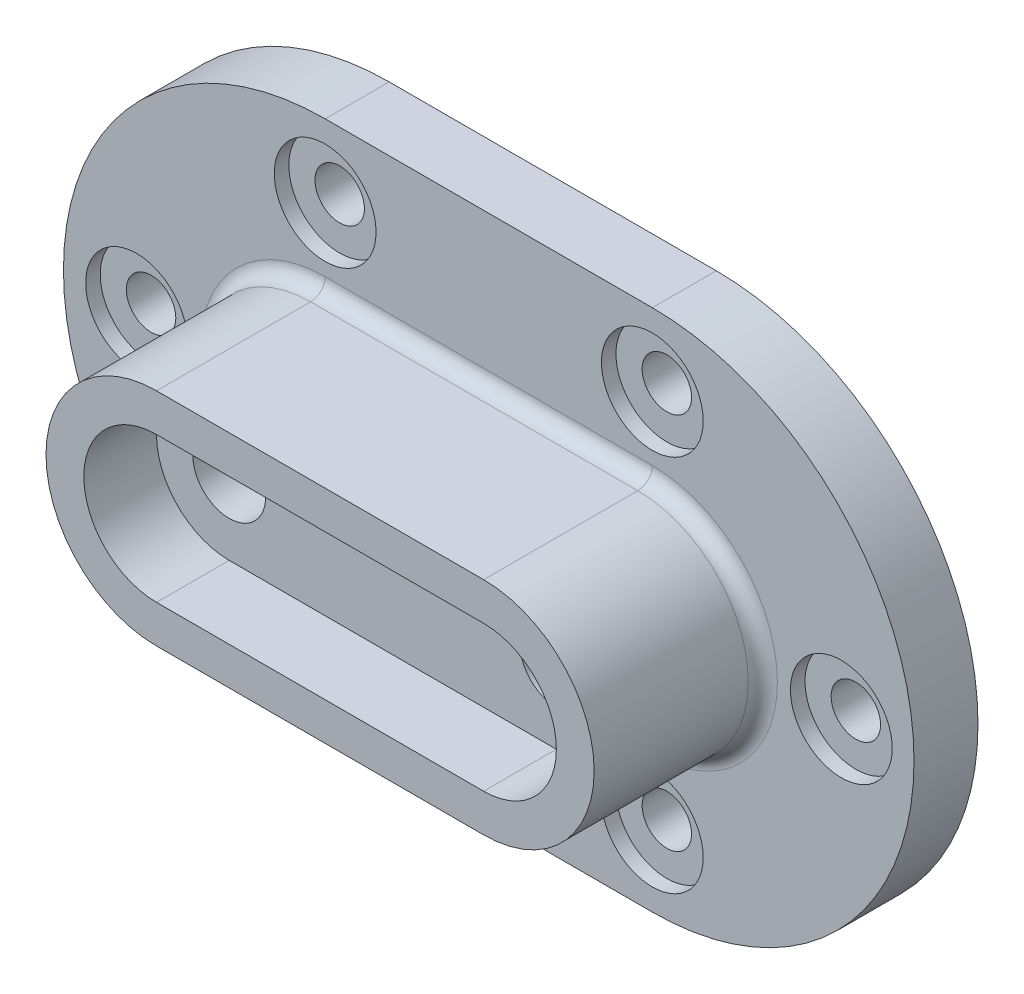
ISO-10303-21;
HEADER;
FILE_DESCRIPTION(('STEP AP214'),'2;1');
FILE_NAME('part.step','',(''),(''),'','','');
FILE_SCHEMA(('AUTOMOTIVE_DESIGN { 1 0 10303 214 1 1 1 1 }'));
ENDSEC;
DATA;
#1=APPLICATION_CONTEXT('core data for automotive mechanical design processes');
#2=APPLICATION_PROTOCOL_DEFINITION('international standard','automotive_design',2000,#1);
#3=PRODUCT_CONTEXT('',#1,'mechanical');
#4=PRODUCT('Part','Part','',(#3));
#5=PRODUCT_RELATED_PRODUCT_CATEGORY('part','',(#4));
#6=PRODUCT_DEFINITION_FORMATION('','',#4);
#7=PRODUCT_DEFINITION_CONTEXT('part definition',#1,'design');
#8=PRODUCT_DEFINITION('design','',#6,#7);
#9=PRODUCT_DEFINITION_SHAPE('','',#8);
#10=(LENGTH_UNIT() NAMED_UNIT(*) SI_UNIT(.MILLI.,.METRE.));
#11=(NAMED_UNIT(*) PLANE_ANGLE_UNIT() SI_UNIT($,.RADIAN.));
#12=(NAMED_UNIT(*) SI_UNIT($,.STERADIAN.) SOLID_ANGLE_UNIT());
#13=UNCERTAINTY_MEASURE_WITH_UNIT(LENGTH_MEASURE(1.E-05),#10,'distance_accuracy_value','');
#14=(GEOMETRIC_REPRESENTATION_CONTEXT(3) GLOBAL_UNCERTAINTY_ASSIGNED_CONTEXT((#13)) GLOBAL_UNIT_ASSIGNED_CONTEXT((#10,
#11,#12)) REPRESENTATION_CONTEXT('',''));
#15=CARTESIAN_POINT('',(0.,0.,0.));
#16=DIRECTION('',(0.,0.,1.));
#17=DIRECTION('',(1.,0.,0.));
#18=AXIS2_PLACEMENT_3D('',#15,#16,#17);
#19=CARTESIAN_POINT('',(-11.25,13.,-0.6));
#20=DIRECTION('',(0.,0.,1.));
#21=DIRECTION('',(1.,0.,0.));
#22=AXIS2_PLACEMENT_3D('',#19,#20,#21);
#23=CYLINDRICAL_SURFACE('',#22,1.7);
#24=CARTESIAN_POINT('',(-11.25,13.,0.));
#25=DIRECTION('',(0.,0.,1.));
#26=DIRECTION('',(1.,0.,0.));
#27=AXIS2_PLACEMENT_3D('',#24,#25,#26);
#28=CIRCLE('',#27,1.7);
#29=CARTESIAN_POINT('',(-9.55000000000004,13.,0.));
#30=VERTEX_POINT('',#29);
#31=EDGE_CURVE('E240',#30,#30,#28,.T.);
#32=ORIENTED_EDGE('',*,*,#31,.F.);
#33=EDGE_LOOP('',(#32));
#34=FACE_BOUND('',#33,.T.);
#35=CARTESIAN_POINT('',(-11.25,13.,3.4));
#36=DIRECTION('',(0.,0.,1.));
#37=DIRECTION('',(1.,0.,0.));
#38=AXIS2_PLACEMENT_3D('',#35,#36,#37);
#39=CIRCLE('',#38,1.7);
#40=CARTESIAN_POINT('',(-9.55000000000004,13.,3.4));
#41=VERTEX_POINT('',#40);
#42=EDGE_CURVE('E243',#41,#41,#39,.F.);
#43=ORIENTED_EDGE('',*,*,#42,.F.);
#44=EDGE_LOOP('',(#43));
#45=FACE_BOUND('',#44,.T.);
#46=ADVANCED_FACE('F39',(#34,#45),#23,.F.);
#47=CARTESIAN_POINT('',(11.2499999999999,13.,-0.6));
#48=DIRECTION('',(0.,0.,1.));
#49=DIRECTION('',(1.,0.,0.));
#50=AXIS2_PLACEMENT_3D('',#47,#48,#49);
#51=CYLINDRICAL_SURFACE('',#50,1.7);
#52=CARTESIAN_POINT('',(11.2499999999999,13.,0.));
#53=DIRECTION('',(0.,0.,1.));
#54=DIRECTION('',(1.,0.,0.));
#55=AXIS2_PLACEMENT_3D('',#52,#53,#54);
#56=CIRCLE('',#55,1.7);
#57=CARTESIAN_POINT('',(12.9499999999999,13.,0.));
#58=VERTEX_POINT('',#57);
#59=EDGE_CURVE('E238',#58,#58,#56,.T.);
#60=ORIENTED_EDGE('',*,*,#59,.F.);
#61=EDGE_LOOP('',(#60));
#62=FACE_BOUND('',#61,.T.);
#63=CARTESIAN_POINT('',(11.2499999999999,13.,3.4));
#64=DIRECTION('',(0.,0.,1.));
#65=DIRECTION('',(1.,0.,0.));
#66=AXIS2_PLACEMENT_3D('',#63,#64,#65);
#67=CIRCLE('',#66,1.7);
#68=CARTESIAN_POINT('',(12.9499999999999,13.,3.4));
#69=VERTEX_POINT('',#68);
#70=EDGE_CURVE('E268',#69,#69,#67,.F.);
#71=ORIENTED_EDGE('',*,*,#70,.F.);
#72=EDGE_LOOP('',(#71));
#73=FACE_BOUND('',#72,.T.);
#74=ADVANCED_FACE('F399',(#62,#73),#51,.F.);
#75=CARTESIAN_POINT('',(24.25,0.,-0.6));
#76=DIRECTION('',(0.,0.,1.));
#77=DIRECTION('',(1.,0.,0.));
#78=AXIS2_PLACEMENT_3D('',#75,#76,#77);
#79=CYLINDRICAL_SURFACE('',#78,1.7);
#80=CARTESIAN_POINT('',(24.25,0.,0.));
#81=DIRECTION('',(0.,0.,1.));
#82=DIRECTION('',(1.,0.,0.));
#83=AXIS2_PLACEMENT_3D('',#80,#81,#82);
#84=CIRCLE('',#83,1.7);
#85=CARTESIAN_POINT('',(25.95,0.,0.));
#86=VERTEX_POINT('',#85);
#87=EDGE_CURVE('E242',#86,#86,#84,.T.);
#88=ORIENTED_EDGE('',*,*,#87,.F.);
#89=EDGE_LOOP('',(#88));
#90=FACE_BOUND('',#89,.T.);
#91=CARTESIAN_POINT('',(24.25,0.,3.4));
#92=DIRECTION('',(0.,0.,1.));
#93=DIRECTION('',(1.,0.,0.));
#94=AXIS2_PLACEMENT_3D('',#91,#92,#93);
#95=CIRCLE('',#94,1.7);
#96=CARTESIAN_POINT('',(25.95,0.,3.4));
#97=VERTEX_POINT('',#96);
#98=EDGE_CURVE('E264',#97,#97,#95,.F.);
#99=ORIENTED_EDGE('',*,*,#98,.F.);
#100=EDGE_LOOP('',(#99));
#101=FACE_BOUND('',#100,.T.);
#102=ADVANCED_FACE('F401',(#90,#101),#79,.F.);
#103=CARTESIAN_POINT('',(11.2500000000001,-13.,-0.6));
#104=DIRECTION('',(0.,0.,1.));
#105=DIRECTION('',(1.,0.,0.));
#106=AXIS2_PLACEMENT_3D('',#103,#104,#105);
#107=CYLINDRICAL_SURFACE('',#106,1.7);
#108=CARTESIAN_POINT('',(11.2500000000001,-13.,0.));
#109=DIRECTION('',(0.,0.,1.));
#110=DIRECTION('',(1.,0.,0.));
#111=AXIS2_PLACEMENT_3D('',#108,#109,#110);
#112=CIRCLE('',#111,1.7);
#113=CARTESIAN_POINT('',(12.9500000000001,-13.,0.));
#114=VERTEX_POINT('',#113);
#115=EDGE_CURVE('E246',#114,#114,#112,.T.);
#116=ORIENTED_EDGE('',*,*,#115,.F.);
#117=EDGE_LOOP('',(#116));
#118=FACE_BOUND('',#117,.T.);
#119=CARTESIAN_POINT('',(11.2500000000001,-13.,3.4));
#120=DIRECTION('',(0.,0.,1.));
#121=DIRECTION('',(1.,0.,0.));
#122=AXIS2_PLACEMENT_3D('',#119,#120,#121);
#123=CIRCLE('',#122,1.7);
#124=CARTESIAN_POINT('',(12.9500000000001,-13.,3.4));
#125=VERTEX_POINT('',#124);
#126=EDGE_CURVE('E265',#125,#125,#123,.F.);
#127=ORIENTED_EDGE('',*,*,#126,.F.);
#128=EDGE_LOOP('',(#127));
#129=FACE_BOUND('',#128,.T.);
#130=ADVANCED_FACE('F413',(#118,#129),#107,.F.);
#131=CARTESIAN_POINT('',(-11.2499999999999,-13.,-0.6));
#132=DIRECTION('',(0.,0.,1.));
#133=DIRECTION('',(1.,0.,0.));
#134=AXIS2_PLACEMENT_3D('',#131,#132,#133);
#135=CYLINDRICAL_SURFACE('',#134,1.7);
#136=CARTESIAN_POINT('',(-11.2499999999999,-13.,0.));
#137=DIRECTION('',(0.,0.,1.));
#138=DIRECTION('',(1.,0.,0.));
#139=AXIS2_PLACEMENT_3D('',#136,#137,#138);
#140=CIRCLE('',#139,1.7);
#141=CARTESIAN_POINT('',(-9.54999999999986,-13.,0.));
#142=VERTEX_POINT('',#141);
#143=EDGE_CURVE('E247',#142,#142,#140,.T.);
#144=ORIENTED_EDGE('',*,*,#143,.F.);
#145=EDGE_LOOP('',(#144));
#146=FACE_BOUND('',#145,.T.);
#147=CARTESIAN_POINT('',(-11.2499999999999,-13.,3.4));
#148=DIRECTION('',(0.,0.,1.));
#149=DIRECTION('',(1.,0.,0.));
#150=AXIS2_PLACEMENT_3D('',#147,#148,#149);
#151=CIRCLE('',#150,1.7);
#152=CARTESIAN_POINT('',(-9.54999999999986,-13.,3.4));
#153=VERTEX_POINT('',#152);
#154=EDGE_CURVE('E256',#153,#153,#151,.F.);
#155=ORIENTED_EDGE('',*,*,#154,.F.);
#156=EDGE_LOOP('',(#155));
#157=FACE_BOUND('',#156,.T.);
#158=ADVANCED_FACE('F407',(#146,#157),#135,.F.);
#159=CARTESIAN_POINT('',(-24.2220429598138,0.,-0.6));
#160=DIRECTION('',(0.,0.,1.));
#161=DIRECTION('',(1.,0.,0.));
#162=AXIS2_PLACEMENT_3D('',#159,#160,#161);
#163=CYLINDRICAL_SURFACE('',#162,1.7);
#164=CARTESIAN_POINT('',(-24.2220429598138,0.,0.));
#165=DIRECTION('',(0.,0.,1.));
#166=DIRECTION('',(1.,0.,0.));
#167=AXIS2_PLACEMENT_3D('',#164,#165,#166);
#168=CIRCLE('',#167,1.7);
#169=CARTESIAN_POINT('',(-22.5220429598138,0.,0.));
#170=VERTEX_POINT('',#169);
#171=EDGE_CURVE('E178',#170,#170,#168,.T.);
#172=ORIENTED_EDGE('',*,*,#171,.F.);
#173=EDGE_LOOP('',(#172));
#174=FACE_BOUND('',#173,.T.);
#175=CARTESIAN_POINT('',(-24.2220429598138,0.,3.4));
#176=DIRECTION('',(0.,0.,1.));
#177=DIRECTION('',(1.,0.,0.));
#178=AXIS2_PLACEMENT_3D('',#175,#176,#177);
#179=CIRCLE('',#178,1.7);
#180=CARTESIAN_POINT('',(-22.5220429598138,0.,3.4));
#181=VERTEX_POINT('',#180);
#182=EDGE_CURVE('E254',#181,#181,#179,.F.);
#183=ORIENTED_EDGE('',*,*,#182,.F.);
#184=EDGE_LOOP('',(#183));
#185=FACE_BOUND('',#184,.T.);
#186=ADVANCED_FACE('F470',(#174,#185),#163,.F.);
#187=CARTESIAN_POINT('',(-11.25,0.,4.4));
#188=DIRECTION('',(0.,0.,-1.));
#189=DIRECTION('',(-1.,0.,0.));
#190=AXIS2_PLACEMENT_3D('',#187,#188,#189);
#191=CYLINDRICAL_SURFACE('',#190,18.);
#192=CARTESIAN_POINT('',(-11.25,0.,0.));
#193=DIRECTION('',(0.,0.,1.));
#194=DIRECTION('',(1.,0.,0.));
#195=AXIS2_PLACEMENT_3D('',#192,#193,#194);
#196=CIRCLE('',#195,18.);
#197=CARTESIAN_POINT('',(-11.25,18.,0.));
#198=VERTEX_POINT('',#197);
#199=CARTESIAN_POINT('',(-11.25,-18.,0.));
#200=VERTEX_POINT('',#199);
#201=EDGE_CURVE('E206',#198,#200,#196,.T.);
#202=ORIENTED_EDGE('',*,*,#201,.T.);
#203=DIRECTION('',(0.,0.,-1.));
#204=VECTOR('',#203,1.);
#205=CARTESIAN_POINT('',(-11.25,-18.,4.4));
#206=LINE('',#205,#204);
#207=CARTESIAN_POINT('',(-11.25,-18.,4.4));
#208=VERTEX_POINT('',#207);
#209=EDGE_CURVE('E235',#208,#200,#206,.T.);
#210=ORIENTED_EDGE('',*,*,#209,.F.);
#211=CARTESIAN_POINT('',(-11.25,0.,4.4));
#212=DIRECTION('',(0.,0.,1.));
#213=DIRECTION('',(1.,0.,0.));
#214=AXIS2_PLACEMENT_3D('',#211,#212,#213);
#215=CIRCLE('',#214,18.);
#216=CARTESIAN_POINT('',(-11.25,18.,4.4));
#217=VERTEX_POINT('',#216);
#218=EDGE_CURVE('E210',#217,#208,#215,.T.);
#219=ORIENTED_EDGE('',*,*,#218,.F.);
#220=DIRECTION('',(0.,0.,-1.));
#221=VECTOR('',#220,1.);
#222=CARTESIAN_POINT('',(-11.25,18.,4.4));
#223=LINE('',#222,#221);
#224=EDGE_CURVE('E220',#217,#198,#223,.T.);
#225=ORIENTED_EDGE('',*,*,#224,.T.);
#226=EDGE_LOOP('',(#202,#210,#219,#225));
#227=FACE_BOUND('',#226,.T.);
#228=ADVANCED_FACE('F366',(#227),#191,.T.);
#229=CARTESIAN_POINT('',(-11.25,-18.,4.4));
#230=DIRECTION('',(0.,1.,0.));
#231=DIRECTION('',(-1.,0.,0.));
#232=AXIS2_PLACEMENT_3D('',#229,#230,#231);
#233=PLANE('',#232);
#234=DIRECTION('',(1.,0.,0.));
#235=VECTOR('',#234,1.);
#236=CARTESIAN_POINT('',(-11.25,-18.,0.));
#237=LINE('',#236,#235);
#238=CARTESIAN_POINT('',(11.25,-18.,0.));
#239=VERTEX_POINT('',#238);
#240=EDGE_CURVE('E219',#200,#239,#237,.T.);
#241=ORIENTED_EDGE('',*,*,#240,.T.);
#242=DIRECTION('',(0.,0.,-1.));
#243=VECTOR('',#242,1.);
#244=CARTESIAN_POINT('',(11.25,-18.,4.4));
#245=LINE('',#244,#243);
#246=CARTESIAN_POINT('',(11.25,-18.,4.4));
#247=VERTEX_POINT('',#246);
#248=EDGE_CURVE('E229',#247,#239,#245,.T.);
#249=ORIENTED_EDGE('',*,*,#248,.F.);
#250=DIRECTION('',(1.,0.,0.));
#251=VECTOR('',#250,1.);
#252=CARTESIAN_POINT('',(-11.25,-18.,4.4));
#253=LINE('',#252,#251);
#254=EDGE_CURVE('E209',#208,#247,#253,.T.);
#255=ORIENTED_EDGE('',*,*,#254,.F.);
#256=ORIENTED_EDGE('',*,*,#209,.T.);
#257=EDGE_LOOP('',(#241,#249,#255,#256));
#258=FACE_BOUND('',#257,.T.);
#259=ADVANCED_FACE('F371',(#258),#233,.F.);
#260=CARTESIAN_POINT('',(11.25,0.,4.4));
#261=DIRECTION('',(0.,0.,-1.));
#262=DIRECTION('',(-1.,0.,0.));
#263=AXIS2_PLACEMENT_3D('',#260,#261,#262);
#264=CYLINDRICAL_SURFACE('',#263,18.);
#265=CARTESIAN_POINT('',(11.25,0.,0.));
#266=DIRECTION('',(0.,0.,1.));
#267=DIRECTION('',(1.,0.,0.));
#268=AXIS2_PLACEMENT_3D('',#265,#266,#267);
#269=CIRCLE('',#268,18.);
#270=CARTESIAN_POINT('',(11.25,18.,0.));
#271=VERTEX_POINT('',#270);
#272=EDGE_CURVE('E225',#239,#271,#269,.T.);
#273=ORIENTED_EDGE('',*,*,#272,.T.);
#274=DIRECTION('',(0.,0.,-1.));
#275=VECTOR('',#274,1.);
#276=CARTESIAN_POINT('',(11.25,18.,4.4));
#277=LINE('',#276,#275);
#278=CARTESIAN_POINT('',(11.25,18.,4.4));
#279=VERTEX_POINT('',#278);
#280=EDGE_CURVE('E230',#279,#271,#277,.T.);
#281=ORIENTED_EDGE('',*,*,#280,.F.);
#282=CARTESIAN_POINT('',(11.25,0.,4.4));
#283=DIRECTION('',(0.,0.,1.));
#284=DIRECTION('',(1.,0.,0.));
#285=AXIS2_PLACEMENT_3D('',#282,#283,#284);
#286=CIRCLE('',#285,18.);
#287=EDGE_CURVE('E213',#247,#279,#286,.T.);
#288=ORIENTED_EDGE('',*,*,#287,.F.);
#289=ORIENTED_EDGE('',*,*,#248,.T.);
#290=EDGE_LOOP('',(#273,#281,#288,#289));
#291=FACE_BOUND('',#290,.T.);
#292=ADVANCED_FACE('F376',(#291),#264,.T.);
#293=CARTESIAN_POINT('',(-11.25,18.,4.4));
#294=DIRECTION('',(0.,-1.,0.));
#295=DIRECTION('',(1.,0.,0.));
#296=AXIS2_PLACEMENT_3D('',#293,#294,#295);
#297=PLANE('',#296);
#298=DIRECTION('',(-1.,0.,0.));
#299=VECTOR('',#298,1.);
#300=CARTESIAN_POINT('',(-11.25,18.,0.));
#301=LINE('',#300,#299);
#302=EDGE_CURVE('E211',#271,#198,#301,.T.);
#303=ORIENTED_EDGE('',*,*,#302,.T.);
#304=ORIENTED_EDGE('',*,*,#224,.F.);
#305=DIRECTION('',(-1.,0.,0.));
#306=VECTOR('',#305,1.);
#307=CARTESIAN_POINT('',(-11.25,18.,4.4));
#308=LINE('',#307,#306);
#309=EDGE_CURVE('E214',#279,#217,#308,.T.);
#310=ORIENTED_EDGE('',*,*,#309,.F.);
#311=ORIENTED_EDGE('',*,*,#280,.T.);
#312=EDGE_LOOP('',(#303,#304,#310,#311));
#313=FACE_BOUND('',#312,.T.);
#314=ADVANCED_FACE('F351',(#313),#297,.F.);
#315=CARTESIAN_POINT('',(-11.25,0.,4.4));
#316=DIRECTION('',(0.,0.,1.));
#317=DIRECTION('',(1.,0.,0.));
#318=AXIS2_PLACEMENT_3D('',#315,#316,#317);
#319=PLANE('',#318);
#320=DIRECTION('',(1.,0.,0.));
#321=VECTOR('',#320,1.);
#322=CARTESIAN_POINT('',(-11.25,-8.6,4.4));
#323=LINE('',#322,#321);
#324=CARTESIAN_POINT('',(11.25,-8.6,4.4));
#325=VERTEX_POINT('',#324);
#326=CARTESIAN_POINT('',(-11.25,-8.6,4.4));
#327=VERTEX_POINT('',#326);
#328=EDGE_CURVE('E274',#325,#327,#323,.F.);
#329=ORIENTED_EDGE('',*,*,#328,.T.);
#330=CARTESIAN_POINT('',(-11.25,0.,4.4));
#331=DIRECTION('',(0.,0.,1.));
#332=DIRECTION('',(1.,0.,0.));
#333=AXIS2_PLACEMENT_3D('',#330,#331,#332);
#334=CIRCLE('',#333,8.6);
#335=CARTESIAN_POINT('',(-11.25,8.6,4.4));
#336=VERTEX_POINT('',#335);
#337=EDGE_CURVE('E283',#327,#336,#334,.F.);
#338=ORIENTED_EDGE('',*,*,#337,.T.);
#339=DIRECTION('',(-1.,0.,0.));
#340=VECTOR('',#339,1.);
#341=CARTESIAN_POINT('',(-11.25,8.6,4.4));
#342=LINE('',#341,#340);
#343=CARTESIAN_POINT('',(11.25,8.6,4.4));
#344=VERTEX_POINT('',#343);
#345=EDGE_CURVE('E276',#336,#344,#342,.F.);
#346=ORIENTED_EDGE('',*,*,#345,.T.);
#347=CARTESIAN_POINT('',(11.25,0.,4.4));
#348=DIRECTION('',(0.,0.,1.));
#349=DIRECTION('',(1.,0.,0.));
#350=AXIS2_PLACEMENT_3D('',#347,#348,#349);
#351=CIRCLE('',#350,8.6);
#352=EDGE_CURVE('E280',#344,#325,#351,.F.);
#353=ORIENTED_EDGE('',*,*,#352,.T.);
#354=EDGE_LOOP('',(#329,#338,#346,#353));
#355=FACE_BOUND('',#354,.T.);
#356=CARTESIAN_POINT('',(-24.2220429598138,0.,4.4));
#357=DIRECTION('',(0.,0.,1.));
#358=DIRECTION('',(1.,0.,0.));
#359=AXIS2_PLACEMENT_3D('',#356,#357,#358);
#360=CIRCLE('',#359,3.5);
#361=CARTESIAN_POINT('',(-20.7220429598138,0.,4.4));
#362=VERTEX_POINT('',#361);
#363=EDGE_CURVE('E311',#362,#362,#360,.T.);
#364=ORIENTED_EDGE('',*,*,#363,.F.);
#365=EDGE_LOOP('',(#364));
#366=FACE_BOUND('',#365,.T.);
#367=CARTESIAN_POINT('',(-11.2499999999999,-13.,4.4));
#368=DIRECTION('',(0.,0.,1.));
#369=DIRECTION('',(1.,0.,0.));
#370=AXIS2_PLACEMENT_3D('',#367,#368,#369);
#371=CIRCLE('',#370,3.5);
#372=CARTESIAN_POINT('',(-7.74999999999986,-13.,4.4));
#373=VERTEX_POINT('',#372);
#374=EDGE_CURVE('E319',#373,#373,#371,.T.);
#375=ORIENTED_EDGE('',*,*,#374,.F.);
#376=EDGE_LOOP('',(#375));
#377=FACE_BOUND('',#376,.T.);
#378=CARTESIAN_POINT('',(11.2500000000001,-13.,4.4));
#379=DIRECTION('',(0.,0.,1.));
#380=DIRECTION('',(1.,0.,0.));
#381=AXIS2_PLACEMENT_3D('',#378,#379,#380);
#382=CIRCLE('',#381,3.5);
#383=CARTESIAN_POINT('',(14.7500000000001,-13.,4.4));
#384=VERTEX_POINT('',#383);
#385=EDGE_CURVE('E175',#384,#384,#382,.T.);
#386=ORIENTED_EDGE('',*,*,#385,.F.);
#387=EDGE_LOOP('',(#386));
#388=FACE_BOUND('',#387,.T.);
#389=CARTESIAN_POINT('',(24.25,0.,4.4));
#390=DIRECTION('',(0.,0.,1.));
#391=DIRECTION('',(1.,0.,0.));
#392=AXIS2_PLACEMENT_3D('',#389,#390,#391);
#393=CIRCLE('',#392,3.5);
#394=CARTESIAN_POINT('',(27.75,0.,4.4));
#395=VERTEX_POINT('',#394);
#396=EDGE_CURVE('E336',#395,#395,#393,.T.);
#397=ORIENTED_EDGE('',*,*,#396,.F.);
#398=EDGE_LOOP('',(#397));
#399=FACE_BOUND('',#398,.T.);
#400=CARTESIAN_POINT('',(11.2499999999999,13.,4.4));
#401=DIRECTION('',(0.,0.,1.));
#402=DIRECTION('',(1.,0.,0.));
#403=AXIS2_PLACEMENT_3D('',#400,#401,#402);
#404=CIRCLE('',#403,3.5);
#405=CARTESIAN_POINT('',(14.7499999999999,13.,4.4));
#406=VERTEX_POINT('',#405);
#407=EDGE_CURVE('E335',#406,#406,#404,.T.);
#408=ORIENTED_EDGE('',*,*,#407,.F.);
#409=EDGE_LOOP('',(#408));
#410=FACE_BOUND('',#409,.T.);
#411=CARTESIAN_POINT('',(-11.25,13.,4.4));
#412=DIRECTION('',(0.,0.,1.));
#413=DIRECTION('',(1.,0.,0.));
#414=AXIS2_PLACEMENT_3D('',#411,#412,#413);
#415=CIRCLE('',#414,3.5);
#416=CARTESIAN_POINT('',(-7.75000000000004,13.,4.4));
#417=VERTEX_POINT('',#416);
#418=EDGE_CURVE('E326',#417,#417,#415,.T.);
#419=ORIENTED_EDGE('',*,*,#418,.F.);
#420=EDGE_LOOP('',(#419));
#421=FACE_BOUND('',#420,.T.);
#422=ORIENTED_EDGE('',*,*,#218,.T.);
#423=ORIENTED_EDGE('',*,*,#254,.T.);
#424=ORIENTED_EDGE('',*,*,#287,.T.);
#425=ORIENTED_EDGE('',*,*,#309,.T.);
#426=EDGE_LOOP('',(#422,#423,#424,#425));
#427=FACE_BOUND('',#426,.T.);
#428=ADVANCED_FACE('F349',(#355,#366,#377,#388,#399,#410,#421,#427),#319,.T.);
#429=CARTESIAN_POINT('',(-11.25,0.,0.));
#430=DIRECTION('',(0.,0.,1.));
#431=DIRECTION('',(1.,0.,0.));
#432=AXIS2_PLACEMENT_3D('',#429,#430,#431);
#433=PLANE('',#432);
#434=CARTESIAN_POINT('',(-11.25,0.,0.));
#435=DIRECTION('',(0.,0.,1.));
#436=DIRECTION('',(1.,0.,0.));
#437=AXIS2_PLACEMENT_3D('',#434,#435,#436);
#438=CIRCLE('',#437,2.5);
#439=CARTESIAN_POINT('',(-8.75,0.,0.));
#440=VERTEX_POINT('',#439);
#441=EDGE_CURVE('E323',#440,#440,#438,.T.);
#442=ORIENTED_EDGE('',*,*,#441,.T.);
#443=EDGE_LOOP('',(#442));
#444=FACE_BOUND('',#443,.T.);
#445=CARTESIAN_POINT('',(11.25,0.,0.));
#446=DIRECTION('',(0.,0.,1.));
#447=DIRECTION('',(1.,0.,0.));
#448=AXIS2_PLACEMENT_3D('',#445,#446,#447);
#449=CIRCLE('',#448,2.5);
#450=CARTESIAN_POINT('',(13.75,0.,0.));
#451=VERTEX_POINT('',#450);
#452=EDGE_CURVE('E301',#451,#451,#449,.T.);
#453=ORIENTED_EDGE('',*,*,#452,.T.);
#454=EDGE_LOOP('',(#453));
#455=FACE_BOUND('',#454,.T.);
#456=ORIENTED_EDGE('',*,*,#171,.T.);
#457=EDGE_LOOP('',(#456));
#458=FACE_BOUND('',#457,.T.);
#459=ORIENTED_EDGE('',*,*,#143,.T.);
#460=EDGE_LOOP('',(#459));
#461=FACE_BOUND('',#460,.T.);
#462=ORIENTED_EDGE('',*,*,#115,.T.);
#463=EDGE_LOOP('',(#462));
#464=FACE_BOUND('',#463,.T.);
#465=ORIENTED_EDGE('',*,*,#87,.T.);
#466=EDGE_LOOP('',(#465));
#467=FACE_BOUND('',#466,.T.);
#468=ORIENTED_EDGE('',*,*,#59,.T.);
#469=EDGE_LOOP('',(#468));
#470=FACE_BOUND('',#469,.T.);
#471=ORIENTED_EDGE('',*,*,#31,.T.);
#472=EDGE_LOOP('',(#471));
#473=FACE_BOUND('',#472,.T.);
#474=ORIENTED_EDGE('',*,*,#201,.F.);
#475=ORIENTED_EDGE('',*,*,#302,.F.);
#476=ORIENTED_EDGE('',*,*,#272,.F.);
#477=ORIENTED_EDGE('',*,*,#240,.F.);
#478=EDGE_LOOP('',(#474,#475,#476,#477));
#479=FACE_BOUND('',#478,.T.);
#480=ADVANCED_FACE('F355',(#444,#455,#458,#461,#464,#467,#470,#473,#479),#433,.F.);
#481=CARTESIAN_POINT('',(-11.25,0.,16.));
#482=DIRECTION('',(0.,0.,-1.));
#483=DIRECTION('',(-1.,0.,0.));
#484=AXIS2_PLACEMENT_3D('',#481,#482,#483);
#485=CYLINDRICAL_SURFACE('',#484,7.6);
#486=DIRECTION('',(0.,0.,-1.));
#487=VECTOR('',#486,1.);
#488=CARTESIAN_POINT('',(-11.25,7.6,16.));
#489=LINE('',#488,#487);
#490=CARTESIAN_POINT('',(-11.25,7.6,16.));
#491=VERTEX_POINT('',#490);
#492=CARTESIAN_POINT('',(-11.25,7.6,5.4));
#493=VERTEX_POINT('',#492);
#494=EDGE_CURVE('E197',#491,#493,#489,.T.);
#495=ORIENTED_EDGE('',*,*,#494,.T.);
#496=CARTESIAN_POINT('',(-11.25,0.,5.4));
#497=DIRECTION('',(0.,0.,1.));
#498=DIRECTION('',(1.,0.,0.));
#499=AXIS2_PLACEMENT_3D('',#496,#497,#498);
#500=CIRCLE('',#499,7.6);
#501=CARTESIAN_POINT('',(-11.25,-7.6,5.4));
#502=VERTEX_POINT('',#501);
#503=EDGE_CURVE('E237',#493,#502,#500,.T.);
#504=ORIENTED_EDGE('',*,*,#503,.T.);
#505=DIRECTION('',(0.,0.,-1.));
#506=VECTOR('',#505,1.);
#507=CARTESIAN_POINT('',(-11.25,-7.6,16.));
#508=LINE('',#507,#506);
#509=CARTESIAN_POINT('',(-11.25,-7.6,16.));
#510=VERTEX_POINT('',#509);
#511=EDGE_CURVE('E204',#510,#502,#508,.T.);
#512=ORIENTED_EDGE('',*,*,#511,.F.);
#513=CARTESIAN_POINT('',(-11.25,0.,16.));
#514=DIRECTION('',(0.,0.,1.));
#515=DIRECTION('',(1.,0.,0.));
#516=AXIS2_PLACEMENT_3D('',#513,#514,#515);
#517=CIRCLE('',#516,7.6);
#518=EDGE_CURVE('E183',#491,#510,#517,.T.);
#519=ORIENTED_EDGE('',*,*,#518,.F.);
#520=EDGE_LOOP('',(#495,#504,#512,#519));
#521=FACE_BOUND('',#520,.T.);
#522=ADVANCED_FACE('F381',(#521),#485,.T.);
#523=CARTESIAN_POINT('',(-11.25,-7.6,16.));
#524=DIRECTION('',(0.,1.,0.));
#525=DIRECTION('',(-1.,0.,0.));
#526=AXIS2_PLACEMENT_3D('',#523,#524,#525);
#527=PLANE('',#526);
#528=ORIENTED_EDGE('',*,*,#511,.T.);
#529=DIRECTION('',(1.,0.,0.));
#530=VECTOR('',#529,1.);
#531=CARTESIAN_POINT('',(-11.25,-7.6,5.4));
#532=LINE('',#531,#530);
#533=CARTESIAN_POINT('',(11.25,-7.6,5.4));
#534=VERTEX_POINT('',#533);
#535=EDGE_CURVE('E11',#502,#534,#532,.T.);
#536=ORIENTED_EDGE('',*,*,#535,.T.);
#537=DIRECTION('',(0.,0.,-1.));
#538=VECTOR('',#537,1.);
#539=CARTESIAN_POINT('',(11.25,-7.6,16.));
#540=LINE('',#539,#538);
#541=CARTESIAN_POINT('',(11.25,-7.6,16.));
#542=VERTEX_POINT('',#541);
#543=EDGE_CURVE('E205',#542,#534,#540,.T.);
#544=ORIENTED_EDGE('',*,*,#543,.F.);
#545=DIRECTION('',(1.,0.,0.));
#546=VECTOR('',#545,1.);
#547=CARTESIAN_POINT('',(-11.25,-7.6,16.));
#548=LINE('',#547,#546);
#549=EDGE_CURVE('E194',#510,#542,#548,.T.);
#550=ORIENTED_EDGE('',*,*,#549,.F.);
#551=EDGE_LOOP('',(#528,#536,#544,#550));
#552=FACE_BOUND('',#551,.T.);
#553=ADVANCED_FACE('F386',(#552),#527,.F.);
#554=CARTESIAN_POINT('',(11.25,0.,16.));
#555=DIRECTION('',(0.,0.,-1.));
#556=DIRECTION('',(-1.,0.,0.));
#557=AXIS2_PLACEMENT_3D('',#554,#555,#556);
#558=CYLINDRICAL_SURFACE('',#557,7.6);
#559=ORIENTED_EDGE('',*,*,#543,.T.);
#560=CARTESIAN_POINT('',(11.25,0.,5.4));
#561=DIRECTION('',(0.,0.,1.));
#562=DIRECTION('',(1.,0.,0.));
#563=AXIS2_PLACEMENT_3D('',#560,#561,#562);
#564=CIRCLE('',#563,7.6);
#565=CARTESIAN_POINT('',(11.25,7.6,5.4));
#566=VERTEX_POINT('',#565);
#567=EDGE_CURVE('E48',#534,#566,#564,.T.);
#568=ORIENTED_EDGE('',*,*,#567,.T.);
#569=DIRECTION('',(0.,0.,-1.));
#570=VECTOR('',#569,1.);
#571=CARTESIAN_POINT('',(11.25,7.6,16.));
#572=LINE('',#571,#570);
#573=CARTESIAN_POINT('',(11.25,7.6,16.));
#574=VERTEX_POINT('',#573);
#575=EDGE_CURVE('E199',#574,#566,#572,.T.);
#576=ORIENTED_EDGE('',*,*,#575,.F.);
#577=CARTESIAN_POINT('',(11.25,0.,16.));
#578=DIRECTION('',(0.,0.,1.));
#579=DIRECTION('',(1.,0.,0.));
#580=AXIS2_PLACEMENT_3D('',#577,#578,#579);
#581=CIRCLE('',#580,7.6);
#582=EDGE_CURVE('E195',#542,#574,#581,.T.);
#583=ORIENTED_EDGE('',*,*,#582,.F.);
#584=EDGE_LOOP('',(#559,#568,#576,#583));
#585=FACE_BOUND('',#584,.T.);
#586=ADVANCED_FACE('F439',(#585),#558,.T.);
#587=CARTESIAN_POINT('',(-11.25,7.6,16.));
#588=DIRECTION('',(0.,-1.,0.));
#589=DIRECTION('',(1.,0.,0.));
#590=AXIS2_PLACEMENT_3D('',#587,#588,#589);
#591=PLANE('',#590);
#592=ORIENTED_EDGE('',*,*,#575,.T.);
#593=DIRECTION('',(-1.,0.,0.));
#594=VECTOR('',#593,1.);
#595=CARTESIAN_POINT('',(-11.25,7.6,5.4));
#596=LINE('',#595,#594);
#597=EDGE_CURVE('E282',#566,#493,#596,.T.);
#598=ORIENTED_EDGE('',*,*,#597,.T.);
#599=ORIENTED_EDGE('',*,*,#494,.F.);
#600=DIRECTION('',(-1.,0.,0.));
#601=VECTOR('',#600,1.);
#602=CARTESIAN_POINT('',(-11.25,7.6,16.));
#603=LINE('',#602,#601);
#604=EDGE_CURVE('E192',#574,#491,#603,.T.);
#605=ORIENTED_EDGE('',*,*,#604,.F.);
#606=EDGE_LOOP('',(#592,#598,#599,#605));
#607=FACE_BOUND('',#606,.T.);
#608=ADVANCED_FACE('F436',(#607),#591,.F.);
#609=CARTESIAN_POINT('',(-11.25,0.,16.));
#610=DIRECTION('',(0.,0.,1.));
#611=DIRECTION('',(1.,0.,0.));
#612=AXIS2_PLACEMENT_3D('',#609,#610,#611);
#613=PLANE('',#612);
#614=CARTESIAN_POINT('',(-11.25,0.,16.));
#615=DIRECTION('',(0.,0.,1.));
#616=DIRECTION('',(1.,0.,0.));
#617=AXIS2_PLACEMENT_3D('',#614,#615,#616);
#618=CIRCLE('',#617,5.);
#619=CARTESIAN_POINT('',(-11.25,5.,16.));
#620=VERTEX_POINT('',#619);
#621=CARTESIAN_POINT('',(-11.25,-5.,16.));
#622=VERTEX_POINT('',#621);
#623=EDGE_CURVE('E149',#620,#622,#618,.T.);
#624=ORIENTED_EDGE('',*,*,#623,.F.);
#625=DIRECTION('',(-1.,0.,0.));
#626=VECTOR('',#625,1.);
#627=CARTESIAN_POINT('',(-11.25,5.,16.));
#628=LINE('',#627,#626);
#629=CARTESIAN_POINT('',(11.25,5.,16.));
#630=VERTEX_POINT('',#629);
#631=EDGE_CURVE('E167',#630,#620,#628,.T.);
#632=ORIENTED_EDGE('',*,*,#631,.F.);
#633=CARTESIAN_POINT('',(11.25,0.,16.));
#634=DIRECTION('',(0.,0.,1.));
#635=DIRECTION('',(1.,0.,0.));
#636=AXIS2_PLACEMENT_3D('',#633,#634,#635);
#637=CIRCLE('',#636,5.);
#638=CARTESIAN_POINT('',(11.25,-5.,16.));
#639=VERTEX_POINT('',#638);
#640=EDGE_CURVE('E166',#639,#630,#637,.T.);
#641=ORIENTED_EDGE('',*,*,#640,.F.);
#642=DIRECTION('',(1.,0.,0.));
#643=VECTOR('',#642,1.);
#644=CARTESIAN_POINT('',(-11.25,-5.,16.));
#645=LINE('',#644,#643);
#646=EDGE_CURVE('E180',#622,#639,#645,.T.);
#647=ORIENTED_EDGE('',*,*,#646,.F.);
#648=EDGE_LOOP('',(#624,#632,#641,#647));
#649=FACE_BOUND('',#648,.T.);
#650=ORIENTED_EDGE('',*,*,#518,.T.);
#651=ORIENTED_EDGE('',*,*,#549,.T.);
#652=ORIENTED_EDGE('',*,*,#582,.T.);
#653=ORIENTED_EDGE('',*,*,#604,.T.);
#654=EDGE_LOOP('',(#650,#651,#652,#653));
#655=FACE_BOUND('',#654,.T.);
#656=ADVANCED_FACE('F433',(#649,#655),#613,.T.);
#657=CARTESIAN_POINT('',(-11.25,0.,11.));
#658=DIRECTION('',(0.,0.,1.));
#659=DIRECTION('',(1.,0.,0.));
#660=AXIS2_PLACEMENT_3D('',#657,#658,#659);
#661=CYLINDRICAL_SURFACE('',#660,5.);
#662=ORIENTED_EDGE('',*,*,#623,.T.);
#663=DIRECTION('',(0.,0.,1.));
#664=VECTOR('',#663,1.);
#665=CARTESIAN_POINT('',(-11.25,-5.,11.));
#666=LINE('',#665,#664);
#667=CARTESIAN_POINT('',(-11.25,-5.,11.));
#668=VERTEX_POINT('',#667);
#669=EDGE_CURVE('E142',#668,#622,#666,.T.);
#670=ORIENTED_EDGE('',*,*,#669,.F.);
#671=CARTESIAN_POINT('',(-11.25,0.,11.));
#672=DIRECTION('',(0.,0.,1.));
#673=DIRECTION('',(1.,0.,0.));
#674=AXIS2_PLACEMENT_3D('',#671,#672,#673);
#675=CIRCLE('',#674,5.);
#676=CARTESIAN_POINT('',(-11.25,5.,11.));
#677=VERTEX_POINT('',#676);
#678=EDGE_CURVE('E148',#677,#668,#675,.T.);
#679=ORIENTED_EDGE('',*,*,#678,.F.);
#680=DIRECTION('',(0.,0.,1.));
#681=VECTOR('',#680,1.);
#682=CARTESIAN_POINT('',(-11.25,5.,11.));
#683=LINE('',#682,#681);
#684=EDGE_CURVE('E181',#677,#620,#683,.T.);
#685=ORIENTED_EDGE('',*,*,#684,.T.);
#686=EDGE_LOOP('',(#662,#670,#679,#685));
#687=FACE_BOUND('',#686,.T.);
#688=ADVANCED_FACE('F145',(#687),#661,.F.);
#689=CARTESIAN_POINT('',(-11.25,5.,11.));
#690=DIRECTION('',(0.,1.,0.));
#691=DIRECTION('',(-1.,0.,0.));
#692=AXIS2_PLACEMENT_3D('',#689,#690,#691);
#693=PLANE('',#692);
#694=ORIENTED_EDGE('',*,*,#631,.T.);
#695=ORIENTED_EDGE('',*,*,#684,.F.);
#696=DIRECTION('',(-1.,0.,0.));
#697=VECTOR('',#696,1.);
#698=CARTESIAN_POINT('',(-11.25,5.,11.));
#699=LINE('',#698,#697);
#700=CARTESIAN_POINT('',(11.25,5.,11.));
#701=VERTEX_POINT('',#700);
#702=EDGE_CURVE('E152',#701,#677,#699,.T.);
#703=ORIENTED_EDGE('',*,*,#702,.F.);
#704=DIRECTION('',(0.,0.,1.));
#705=VECTOR('',#704,1.);
#706=CARTESIAN_POINT('',(11.25,5.,11.));
#707=LINE('',#706,#705);
#708=EDGE_CURVE('E188',#701,#630,#707,.T.);
#709=ORIENTED_EDGE('',*,*,#708,.T.);
#710=EDGE_LOOP('',(#694,#695,#703,#709));
#711=FACE_BOUND('',#710,.T.);
#712=ADVANCED_FACE('F425',(#711),#693,.F.);
#713=CARTESIAN_POINT('',(11.25,0.,11.));
#714=DIRECTION('',(0.,0.,1.));
#715=DIRECTION('',(1.,0.,0.));
#716=AXIS2_PLACEMENT_3D('',#713,#714,#715);
#717=CYLINDRICAL_SURFACE('',#716,5.);
#718=ORIENTED_EDGE('',*,*,#640,.T.);
#719=ORIENTED_EDGE('',*,*,#708,.F.);
#720=CARTESIAN_POINT('',(11.25,0.,11.));
#721=DIRECTION('',(0.,0.,1.));
#722=DIRECTION('',(1.,0.,0.));
#723=AXIS2_PLACEMENT_3D('',#720,#721,#722);
#724=CIRCLE('',#723,5.);
#725=CARTESIAN_POINT('',(11.25,-5.,11.));
#726=VERTEX_POINT('',#725);
#727=EDGE_CURVE('E165',#726,#701,#724,.T.);
#728=ORIENTED_EDGE('',*,*,#727,.F.);
#729=DIRECTION('',(0.,0.,1.));
#730=VECTOR('',#729,1.);
#731=CARTESIAN_POINT('',(11.25,-5.,11.));
#732=LINE('',#731,#730);
#733=EDGE_CURVE('E153',#726,#639,#732,.T.);
#734=ORIENTED_EDGE('',*,*,#733,.T.);
#735=EDGE_LOOP('',(#718,#719,#728,#734));
#736=FACE_BOUND('',#735,.T.);
#737=ADVANCED_FACE('F422',(#736),#717,.F.);
#738=CARTESIAN_POINT('',(-11.25,-5.,11.));
#739=DIRECTION('',(0.,-1.,0.));
#740=DIRECTION('',(1.,0.,0.));
#741=AXIS2_PLACEMENT_3D('',#738,#739,#740);
#742=PLANE('',#741);
#743=ORIENTED_EDGE('',*,*,#646,.T.);
#744=ORIENTED_EDGE('',*,*,#733,.F.);
#745=DIRECTION('',(1.,0.,0.));
#746=VECTOR('',#745,1.);
#747=CARTESIAN_POINT('',(-11.25,-5.,11.));
#748=LINE('',#747,#746);
#749=EDGE_CURVE('E160',#668,#726,#748,.T.);
#750=ORIENTED_EDGE('',*,*,#749,.F.);
#751=ORIENTED_EDGE('',*,*,#669,.T.);
#752=EDGE_LOOP('',(#743,#744,#750,#751));
#753=FACE_BOUND('',#752,.T.);
#754=ADVANCED_FACE('F158',(#753),#742,.F.);
#755=CARTESIAN_POINT('',(-11.25,0.,11.));
#756=DIRECTION('',(0.,0.,1.));
#757=DIRECTION('',(1.,0.,0.));
#758=AXIS2_PLACEMENT_3D('',#755,#756,#757);
#759=PLANE('',#758);
#760=CARTESIAN_POINT('',(-11.25,0.,11.));
#761=DIRECTION('',(0.,0.,1.));
#762=DIRECTION('',(1.,0.,0.));
#763=AXIS2_PLACEMENT_3D('',#760,#761,#762);
#764=CIRCLE('',#763,2.5);
#765=CARTESIAN_POINT('',(-8.75,0.,11.));
#766=VERTEX_POINT('',#765);
#767=EDGE_CURVE('E307',#766,#766,#764,.T.);
#768=ORIENTED_EDGE('',*,*,#767,.F.);
#769=EDGE_LOOP('',(#768));
#770=FACE_BOUND('',#769,.T.);
#771=CARTESIAN_POINT('',(11.25,0.,11.));
#772=DIRECTION('',(0.,0.,1.));
#773=DIRECTION('',(1.,0.,0.));
#774=AXIS2_PLACEMENT_3D('',#771,#772,#773);
#775=CIRCLE('',#774,2.5);
#776=CARTESIAN_POINT('',(13.75,0.,11.));
#777=VERTEX_POINT('',#776);
#778=EDGE_CURVE('E298',#777,#777,#775,.T.);
#779=ORIENTED_EDGE('',*,*,#778,.F.);
#780=EDGE_LOOP('',(#779));
#781=FACE_BOUND('',#780,.T.);
#782=ORIENTED_EDGE('',*,*,#678,.T.);
#783=ORIENTED_EDGE('',*,*,#749,.T.);
#784=ORIENTED_EDGE('',*,*,#727,.T.);
#785=ORIENTED_EDGE('',*,*,#702,.T.);
#786=EDGE_LOOP('',(#782,#783,#784,#785));
#787=FACE_BOUND('',#786,.T.);
#788=ADVANCED_FACE('F163',(#770,#781,#787),#759,.T.);
#789=CARTESIAN_POINT('',(-24.2220429598138,0.,3.4));
#790=DIRECTION('',(0.,0.,1.));
#791=DIRECTION('',(1.,0.,0.));
#792=AXIS2_PLACEMENT_3D('',#789,#790,#791);
#793=PLANE('',#792);
#794=CARTESIAN_POINT('',(-24.2220429598138,0.,3.4));
#795=DIRECTION('',(0.,0.,1.));
#796=DIRECTION('',(1.,0.,0.));
#797=AXIS2_PLACEMENT_3D('',#794,#795,#796);
#798=CIRCLE('',#797,3.5);
#799=CARTESIAN_POINT('',(-20.7220429598138,0.,3.4));
#800=VERTEX_POINT('',#799);
#801=EDGE_CURVE('E259',#800,#800,#798,.T.);
#802=ORIENTED_EDGE('',*,*,#801,.T.);
#803=EDGE_LOOP('',(#802));
#804=FACE_BOUND('',#803,.T.);
#805=ORIENTED_EDGE('',*,*,#182,.T.);
#806=EDGE_LOOP('',(#805));
#807=FACE_BOUND('',#806,.T.);
#808=ADVANCED_FACE('F419',(#804,#807),#793,.T.);
#809=CARTESIAN_POINT('',(-24.2220429598138,0.,3.4));
#810=DIRECTION('',(0.,0.,1.));
#811=DIRECTION('',(1.,0.,0.));
#812=AXIS2_PLACEMENT_3D('',#809,#810,#811);
#813=CYLINDRICAL_SURFACE('',#812,3.5);
#814=ORIENTED_EDGE('',*,*,#801,.F.);
#815=EDGE_LOOP('',(#814));
#816=FACE_BOUND('',#815,.T.);
#817=ORIENTED_EDGE('',*,*,#363,.T.);
#818=EDGE_LOOP('',(#817));
#819=FACE_BOUND('',#818,.T.);
#820=ADVANCED_FACE('F551',(#816,#819),#813,.F.);
#821=CARTESIAN_POINT('',(-11.2499999999999,-13.,3.4));
#822=DIRECTION('',(0.,0.,1.));
#823=DIRECTION('',(1.,0.,0.));
#824=AXIS2_PLACEMENT_3D('',#821,#822,#823);
#825=PLANE('',#824);
#826=CARTESIAN_POINT('',(-11.2499999999999,-13.,3.4));
#827=DIRECTION('',(0.,0.,1.));
#828=DIRECTION('',(1.,0.,0.));
#829=AXIS2_PLACEMENT_3D('',#826,#827,#828);
#830=CIRCLE('',#829,3.5);
#831=CARTESIAN_POINT('',(-7.74999999999986,-13.,3.4));
#832=VERTEX_POINT('',#831);
#833=EDGE_CURVE('E320',#832,#832,#830,.T.);
#834=ORIENTED_EDGE('',*,*,#833,.T.);
#835=EDGE_LOOP('',(#834));
#836=FACE_BOUND('',#835,.T.);
#837=ORIENTED_EDGE('',*,*,#154,.T.);
#838=EDGE_LOOP('',(#837));
#839=FACE_BOUND('',#838,.T.);
#840=ADVANCED_FACE('F563',(#836,#839),#825,.T.);
#841=CARTESIAN_POINT('',(-11.2499999999999,-13.,3.4));
#842=DIRECTION('',(0.,0.,1.));
#843=DIRECTION('',(1.,0.,0.));
#844=AXIS2_PLACEMENT_3D('',#841,#842,#843);
#845=CYLINDRICAL_SURFACE('',#844,3.5);
#846=ORIENTED_EDGE('',*,*,#833,.F.);
#847=EDGE_LOOP('',(#846));
#848=FACE_BOUND('',#847,.T.);
#849=ORIENTED_EDGE('',*,*,#374,.T.);
#850=EDGE_LOOP('',(#849));
#851=FACE_BOUND('',#850,.T.);
#852=ADVANCED_FACE('F572',(#848,#851),#845,.F.);
#853=CARTESIAN_POINT('',(11.2500000000001,-13.,3.4));
#854=DIRECTION('',(0.,0.,1.));
#855=DIRECTION('',(1.,0.,0.));
#856=AXIS2_PLACEMENT_3D('',#853,#854,#855);
#857=PLANE('',#856);
#858=CARTESIAN_POINT('',(11.2500000000001,-13.,3.4));
#859=DIRECTION('',(0.,0.,1.));
#860=DIRECTION('',(1.,0.,0.));
#861=AXIS2_PLACEMENT_3D('',#858,#859,#860);
#862=CIRCLE('',#861,3.5);
#863=CARTESIAN_POINT('',(14.7500000000001,-13.,3.4));
#864=VERTEX_POINT('',#863);
#865=EDGE_CURVE('E339',#864,#864,#862,.T.);
#866=ORIENTED_EDGE('',*,*,#865,.T.);
#867=EDGE_LOOP('',(#866));
#868=FACE_BOUND('',#867,.T.);
#869=ORIENTED_EDGE('',*,*,#126,.T.);
#870=EDGE_LOOP('',(#869));
#871=FACE_BOUND('',#870,.T.);
#872=ADVANCED_FACE('F585',(#868,#871),#857,.T.);
#873=CARTESIAN_POINT('',(11.2500000000001,-13.,3.4));
#874=DIRECTION('',(0.,0.,1.));
#875=DIRECTION('',(1.,0.,0.));
#876=AXIS2_PLACEMENT_3D('',#873,#874,#875);
#877=CYLINDRICAL_SURFACE('',#876,3.5);
#878=ORIENTED_EDGE('',*,*,#865,.F.);
#879=EDGE_LOOP('',(#878));
#880=FACE_BOUND('',#879,.T.);
#881=ORIENTED_EDGE('',*,*,#385,.T.);
#882=EDGE_LOOP('',(#881));
#883=FACE_BOUND('',#882,.T.);
#884=ADVANCED_FACE('F350',(#880,#883),#877,.F.);
#885=CARTESIAN_POINT('',(24.25,0.,3.4));
#886=DIRECTION('',(0.,0.,1.));
#887=DIRECTION('',(1.,0.,0.));
#888=AXIS2_PLACEMENT_3D('',#885,#886,#887);
#889=PLANE('',#888);
#890=CARTESIAN_POINT('',(24.25,0.,3.4));
#891=DIRECTION('',(0.,0.,1.));
#892=DIRECTION('',(1.,0.,0.));
#893=AXIS2_PLACEMENT_3D('',#890,#891,#892);
#894=CIRCLE('',#893,3.5);
#895=CARTESIAN_POINT('',(27.75,0.,3.4));
#896=VERTEX_POINT('',#895);
#897=EDGE_CURVE('E333',#896,#896,#894,.T.);
#898=ORIENTED_EDGE('',*,*,#897,.T.);
#899=EDGE_LOOP('',(#898));
#900=FACE_BOUND('',#899,.T.);
#901=ORIENTED_EDGE('',*,*,#98,.T.);
#902=EDGE_LOOP('',(#901));
#903=FACE_BOUND('',#902,.T.);
#904=ADVANCED_FACE('F605',(#900,#903),#889,.T.);
#905=CARTESIAN_POINT('',(24.25,0.,3.4));
#906=DIRECTION('',(0.,0.,1.));
#907=DIRECTION('',(1.,0.,0.));
#908=AXIS2_PLACEMENT_3D('',#905,#906,#907);
#909=CYLINDRICAL_SURFACE('',#908,3.5);
#910=ORIENTED_EDGE('',*,*,#897,.F.);
#911=EDGE_LOOP('',(#910));
#912=FACE_BOUND('',#911,.T.);
#913=ORIENTED_EDGE('',*,*,#396,.T.);
#914=EDGE_LOOP('',(#913));
#915=FACE_BOUND('',#914,.T.);
#916=ADVANCED_FACE('F615',(#912,#915),#909,.F.);
#917=CARTESIAN_POINT('',(11.2499999999999,13.,3.4));
#918=DIRECTION('',(0.,0.,1.));
#919=DIRECTION('',(1.,0.,0.));
#920=AXIS2_PLACEMENT_3D('',#917,#918,#919);
#921=PLANE('',#920);
#922=CARTESIAN_POINT('',(11.2499999999999,13.,3.4));
#923=DIRECTION('',(0.,0.,1.));
#924=DIRECTION('',(1.,0.,0.));
#925=AXIS2_PLACEMENT_3D('',#922,#923,#924);
#926=CIRCLE('',#925,3.5);
#927=CARTESIAN_POINT('',(14.7499999999999,13.,3.4));
#928=VERTEX_POINT('',#927);
#929=EDGE_CURVE('E328',#928,#928,#926,.T.);
#930=ORIENTED_EDGE('',*,*,#929,.T.);
#931=EDGE_LOOP('',(#930));
#932=FACE_BOUND('',#931,.T.);
#933=ORIENTED_EDGE('',*,*,#70,.T.);
#934=EDGE_LOOP('',(#933));
#935=FACE_BOUND('',#934,.T.);
#936=ADVANCED_FACE('F625',(#932,#935),#921,.T.);
#937=CARTESIAN_POINT('',(11.2499999999999,13.,3.4));
#938=DIRECTION('',(0.,0.,1.));
#939=DIRECTION('',(1.,0.,0.));
#940=AXIS2_PLACEMENT_3D('',#937,#938,#939);
#941=CYLINDRICAL_SURFACE('',#940,3.5);
#942=ORIENTED_EDGE('',*,*,#929,.F.);
#943=EDGE_LOOP('',(#942));
#944=FACE_BOUND('',#943,.T.);
#945=ORIENTED_EDGE('',*,*,#407,.T.);
#946=EDGE_LOOP('',(#945));
#947=FACE_BOUND('',#946,.T.);
#948=ADVANCED_FACE('F631',(#944,#947),#941,.F.);
#949=CARTESIAN_POINT('',(-11.25,13.,3.4));
#950=DIRECTION('',(0.,0.,1.));
#951=DIRECTION('',(1.,0.,0.));
#952=AXIS2_PLACEMENT_3D('',#949,#950,#951);
#953=PLANE('',#952);
#954=CARTESIAN_POINT('',(-11.25,13.,3.4));
#955=DIRECTION('',(0.,0.,1.));
#956=DIRECTION('',(1.,0.,0.));
#957=AXIS2_PLACEMENT_3D('',#954,#955,#956);
#958=CIRCLE('',#957,3.5);
#959=CARTESIAN_POINT('',(-7.75000000000004,13.,3.4));
#960=VERTEX_POINT('',#959);
#961=EDGE_CURVE('E316',#960,#960,#958,.T.);
#962=ORIENTED_EDGE('',*,*,#961,.T.);
#963=EDGE_LOOP('',(#962));
#964=FACE_BOUND('',#963,.T.);
#965=ORIENTED_EDGE('',*,*,#42,.T.);
#966=EDGE_LOOP('',(#965));
#967=FACE_BOUND('',#966,.T.);
#968=ADVANCED_FACE('F645',(#964,#967),#953,.T.);
#969=CARTESIAN_POINT('',(-11.25,13.,3.4));
#970=DIRECTION('',(0.,0.,1.));
#971=DIRECTION('',(1.,0.,0.));
#972=AXIS2_PLACEMENT_3D('',#969,#970,#971);
#973=CYLINDRICAL_SURFACE('',#972,3.5);
#974=ORIENTED_EDGE('',*,*,#961,.F.);
#975=EDGE_LOOP('',(#974));
#976=FACE_BOUND('',#975,.T.);
#977=ORIENTED_EDGE('',*,*,#418,.T.);
#978=EDGE_LOOP('',(#977));
#979=FACE_BOUND('',#978,.T.);
#980=ADVANCED_FACE('F655',(#976,#979),#973,.F.);
#981=CARTESIAN_POINT('',(11.25,0.,0.));
#982=DIRECTION('',(0.,0.,1.));
#983=DIRECTION('',(1.,0.,0.));
#984=AXIS2_PLACEMENT_3D('',#981,#982,#983);
#985=CYLINDRICAL_SURFACE('',#984,2.5);
#986=ORIENTED_EDGE('',*,*,#452,.F.);
#987=EDGE_LOOP('',(#986));
#988=FACE_BOUND('',#987,.T.);
#989=ORIENTED_EDGE('',*,*,#778,.T.);
#990=EDGE_LOOP('',(#989));
#991=FACE_BOUND('',#990,.T.);
#992=ADVANCED_FACE('F662',(#988,#991),#985,.F.);
#993=CARTESIAN_POINT('',(-11.25,0.,0.));
#994=DIRECTION('',(0.,0.,1.));
#995=DIRECTION('',(1.,0.,0.));
#996=AXIS2_PLACEMENT_3D('',#993,#994,#995);
#997=CYLINDRICAL_SURFACE('',#996,2.5);
#998=ORIENTED_EDGE('',*,*,#441,.F.);
#999=EDGE_LOOP('',(#998));
#1000=FACE_BOUND('',#999,.T.);
#1001=ORIENTED_EDGE('',*,*,#767,.T.);
#1002=EDGE_LOOP('',(#1001));
#1003=FACE_BOUND('',#1002,.T.);
#1004=ADVANCED_FACE('F669',(#1000,#1003),#997,.F.);
#1005=CARTESIAN_POINT('',(11.25,0.,5.4));
#1006=DIRECTION('',(0.,0.,1.));
#1007=DIRECTION('',(1.,0.,0.));
#1008=AXIS2_PLACEMENT_3D('',#1005,#1006,#1007);
#1009=TOROIDAL_SURFACE('',#1008,8.6,1.);
#1010=CARTESIAN_POINT('',(11.25,-8.6,5.4));
#1011=DIRECTION('',(1.,0.,0.));
#1012=DIRECTION('',(0.,0.,-1.));
#1013=AXIS2_PLACEMENT_3D('',#1010,#1011,#1012);
#1014=CIRCLE('',#1013,1.);
#1015=EDGE_CURVE('E287',#325,#534,#1014,.T.);
#1016=ORIENTED_EDGE('',*,*,#1015,.F.);
#1017=ORIENTED_EDGE('',*,*,#352,.F.);
#1018=CARTESIAN_POINT('',(11.25,8.6,5.4));
#1019=DIRECTION('',(1.,0.,0.));
#1020=DIRECTION('',(0.,0.,-1.));
#1021=AXIS2_PLACEMENT_3D('',#1018,#1019,#1020);
#1022=CIRCLE('',#1021,1.);
#1023=EDGE_CURVE('E43',#566,#344,#1022,.T.);
#1024=ORIENTED_EDGE('',*,*,#1023,.F.);
#1025=ORIENTED_EDGE('',*,*,#567,.F.);
#1026=EDGE_LOOP('',(#1016,#1017,#1024,#1025));
#1027=FACE_BOUND('',#1026,.T.);
#1028=ADVANCED_FACE('F41',(#1027),#1009,.F.);
#1029=CARTESIAN_POINT('',(-11.25,8.6,5.4));
#1030=DIRECTION('',(-1.,0.,0.));
#1031=DIRECTION('',(0.,-1.,0.));
#1032=AXIS2_PLACEMENT_3D('',#1029,#1030,#1031);
#1033=CYLINDRICAL_SURFACE('',#1032,1.);
#1034=ORIENTED_EDGE('',*,*,#1023,.T.);
#1035=ORIENTED_EDGE('',*,*,#345,.F.);
#1036=CARTESIAN_POINT('',(-11.25,8.6,5.4));
#1037=DIRECTION('',(1.,0.,0.));
#1038=DIRECTION('',(0.,0.,-1.));
#1039=AXIS2_PLACEMENT_3D('',#1036,#1037,#1038);
#1040=CIRCLE('',#1039,1.);
#1041=EDGE_CURVE('E288',#493,#336,#1040,.T.);
#1042=ORIENTED_EDGE('',*,*,#1041,.F.);
#1043=ORIENTED_EDGE('',*,*,#597,.F.);
#1044=EDGE_LOOP('',(#1034,#1035,#1042,#1043));
#1045=FACE_BOUND('',#1044,.T.);
#1046=ADVANCED_FACE('F456',(#1045),#1033,.F.);
#1047=CARTESIAN_POINT('',(-11.25,-8.6,5.4));
#1048=DIRECTION('',(1.,0.,0.));
#1049=DIRECTION('',(0.,1.,0.));
#1050=AXIS2_PLACEMENT_3D('',#1047,#1048,#1049);
#1051=CYLINDRICAL_SURFACE('',#1050,1.);
#1052=ORIENTED_EDGE('',*,*,#1015,.T.);
#1053=ORIENTED_EDGE('',*,*,#535,.F.);
#1054=CARTESIAN_POINT('',(-11.25,-8.6,5.4));
#1055=DIRECTION('',(1.,0.,0.));
#1056=DIRECTION('',(0.,0.,-1.));
#1057=AXIS2_PLACEMENT_3D('',#1054,#1055,#1056);
#1058=CIRCLE('',#1057,1.);
#1059=EDGE_CURVE('E286',#327,#502,#1058,.T.);
#1060=ORIENTED_EDGE('',*,*,#1059,.F.);
#1061=ORIENTED_EDGE('',*,*,#328,.F.);
#1062=EDGE_LOOP('',(#1052,#1053,#1060,#1061));
#1063=FACE_BOUND('',#1062,.T.);
#1064=ADVANCED_FACE('F457',(#1063),#1051,.F.);
#1065=CARTESIAN_POINT('',(-11.25,0.,5.4));
#1066=DIRECTION('',(0.,0.,1.));
#1067=DIRECTION('',(1.,0.,0.));
#1068=AXIS2_PLACEMENT_3D('',#1065,#1066,#1067);
#1069=TOROIDAL_SURFACE('',#1068,8.6,1.);
#1070=ORIENTED_EDGE('',*,*,#1041,.T.);
#1071=ORIENTED_EDGE('',*,*,#337,.F.);
#1072=ORIENTED_EDGE('',*,*,#1059,.T.);
#1073=ORIENTED_EDGE('',*,*,#503,.F.);
#1074=EDGE_LOOP('',(#1070,#1071,#1072,#1073));
#1075=FACE_BOUND('',#1074,.T.);
#1076=ADVANCED_FACE('F455',(#1075),#1069,.F.);
#1077=CLOSED_SHELL('',(#46,#74,#102,#130,#158,#186,#228,#259,#292,#314,#428,#480,#522,#553,#586,
#608,#656,#688,#712,#737,#754,#788,#808,#820,#840,#852,#872,#884,#904,#916,#936,#948,#968,#980,
#992,#1004,#1028,#1046,#1064,#1076));
#1078=MANIFOLD_SOLID_BREP('B2',#1077);
#1079=ADVANCED_BREP_SHAPE_REPRESENTATION('',(#18,#1078),#14);
#1080=SHAPE_DEFINITION_REPRESENTATION(#9,#1079);
ENDSEC;
END-ISO-10303-21;
